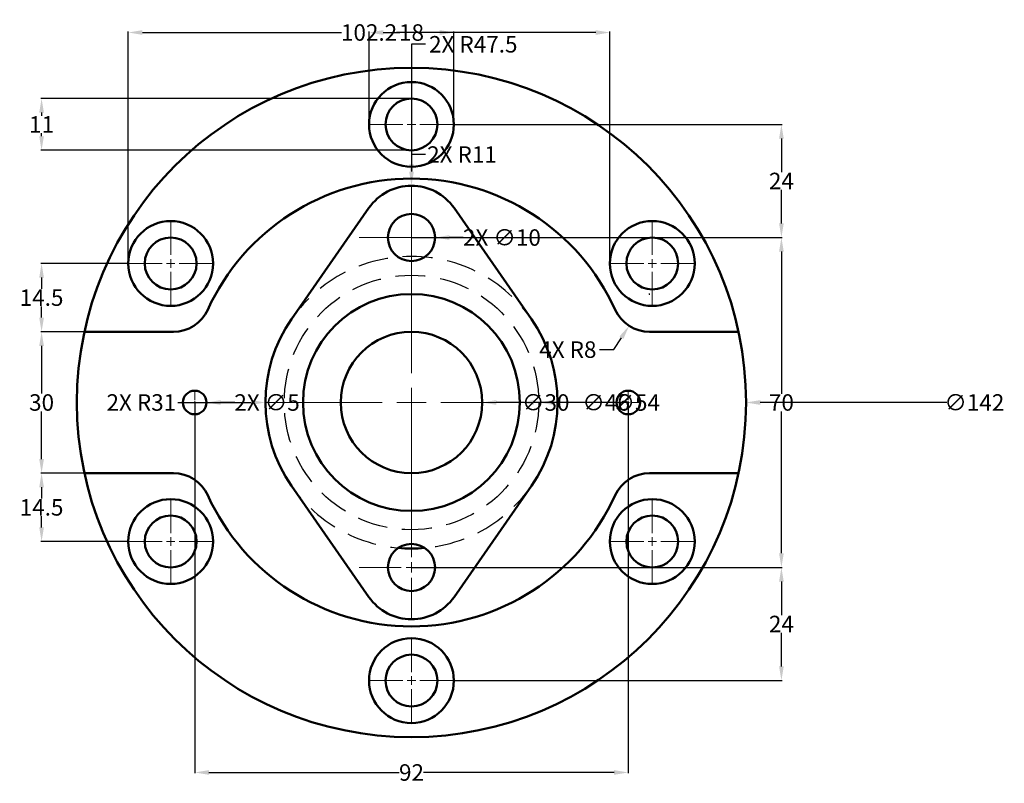
# Model space of a CAD drawing. Units: millimetres. Extents: x 646 to 860, y 238 to 552.
# Tile 2 of 2: x 651 to 860, y 390 to 552. Entities that reach past the tile are written whole.
import ezdxf

# ---------------------------------------------------------------- set-up
doc = ezdxf.new("R2010")
doc.units = ezdxf.units.MM
doc.header["$MEASUREMENT"] = 0
doc.linetypes.add('CENTER', pattern=[50.8, 31.75, -6.35, 6.35, -6.35])
doc.linetypes.add('HIDDEN', pattern=[9.525, 6.35, -3.175])
for name, color, linetype, lineweight in [('M-CNTR', 1, 'CENTER', 18), ('M-DIMS', 2, 'Continuous', 18), ('M-HIDN', 4, 'HIDDEN', 25), ('M-OUTL', 7, 'Continuous', 50)]:
    doc.layers.add(name, color=color, linetype=linetype, lineweight=lineweight)
doc.styles.get("Standard").update_dxf_attribs({"font": 'arial.ttf'})
doc.dimstyles.get("Standard").update_dxf_attribs({"dimtxt": 3.5, "dimasz": 3, "dimexe": 0.18, "dimexo": 0.0625, "dimgap": 0.09, "dimtad": 0, "dimtih": 1, "dimtoh": 1, "dimdec": 1, "dimzin": 0, "dimdsep": 46, "dimtxsty": 'Standard', "dimcen": 0.09, "dimadec": 0, "dimazin": 0, "dimtfac": 1, "dimtdec": 1, "dimtofl": 0, "dimtmove": 0, "dimatfit": 3, "dimfxl": 1, "dimtolj": 1, "dimtzin": 0, "dimarcsym": 0})

# ---------------------------------------------------------------- blocks, each defined once
blk = doc.blocks.new('*U1')
for radius in [9, 5.5]:
    blk.add_circle((0, 0), radius)
blk = doc.blocks.new('*U2')
at = {"layer": 'M-OUTL', "color": 0, "linetype": 'ByBlock', "lineweight": -2, "transparency": 16777216}
blk.add_blockref('*U1', (191, 167.28), dxfattribs=at)
for p, rotation in [((139.9, 137.78), 59.99999999999999), ((242.1, 137.78), 300), ((139.9, 78.78), 120), ((242.1, 78.78), 240), ((191, 49.28), 180)]:
    blk.add_blockref('*U1', p, dxfattribs=dict(at, rotation=rotation))
blk = doc.blocks.new('*U3')
at = {"layer": 'M-CNTR', "color": 0, "transparency": 16777216}
for p, q in [((0, 1.8), (0, 9.12)), ((-9.12, 0), (-1.8, 0)), ((1.8, 0), (9.12, 0)), ((0, -9.12), (0, -1.8))]:
    blk.add_line(p, q, dxfattribs=at)
at = {"layer": 'M-CNTR', "color": 0, "linetype": 'Continuous', "transparency": 16777216}
for p, q in [((-0.9, 0), (0.9, 0)), ((0, -0.9), (0, 0.9))]:
    blk.add_line(p, q, dxfattribs=at)
blk = doc.blocks.new('*U4')
at = {"layer": 'M-CNTR', "color": 0, "transparency": 16777216}
for p, q in [((0, 1.8), (0, 9.12)), ((-9.12, 0), (-1.8, 0)), ((1.8, 0), (9.12, 0)), ((0, -9.12), (0, -1.8))]:
    blk.add_line(p, q, dxfattribs=at)
at = {"layer": 'M-CNTR', "color": 0, "linetype": 'Continuous', "transparency": 16777216}
for p, q in [((-0.9, 0), (0.9, 0)), ((0, -0.9), (0, 0.9))]:
    blk.add_line(p, q, dxfattribs=at)
blk = doc.blocks.new('*U5')
at = {"layer": 'M-CNTR', "color": 0, "transparency": 16777216}
for p, q in [((0, 1.8), (0, 9.12)), ((-9.12, 0), (-1.8, 0)), ((1.8, 0), (9.12, 0)), ((0, -9.12), (0, -1.8))]:
    blk.add_line(p, q, dxfattribs=at)
at = {"layer": 'M-CNTR', "color": 0, "linetype": 'Continuous', "transparency": 16777216}
for p, q in [((-0.9, 0), (0.9, 0)), ((0, -0.9), (0, 0.9))]:
    blk.add_line(p, q, dxfattribs=at)
blk = doc.blocks.new('*U6')
at = {"layer": 'M-CNTR', "color": 0, "transparency": 16777216}
for p, q in [((0, 1.8), (0, 9.12)), ((-9.12, 0), (-1.8, 0)), ((1.8, 0), (9.12, 0)), ((0, -9.12), (0, -1.8))]:
    blk.add_line(p, q, dxfattribs=at)
at = {"layer": 'M-CNTR', "color": 0, "linetype": 'Continuous', "transparency": 16777216}
for p, q in [((-0.9, 0), (0.9, 0)), ((0, -0.9), (0, 0.9))]:
    blk.add_line(p, q, dxfattribs=at)
blk = doc.blocks.new('*U7')
at = {"layer": 'M-CNTR', "color": 0, "transparency": 16777216}
for p, q in [((0, 1.8), (0, 9.12)), ((-9.12, 0), (-1.8, 0)), ((1.8, 0), (9.12, 0)), ((0, -9.12), (0, -1.8))]:
    blk.add_line(p, q, dxfattribs=at)
at = {"layer": 'M-CNTR', "color": 0, "linetype": 'Continuous', "transparency": 16777216}
for p, q in [((-0.9, 0), (0.9, 0)), ((0, -0.9), (0, 0.9))]:
    blk.add_line(p, q, dxfattribs=at)
blk = doc.blocks.new('*U8')
at = {"layer": 'M-CNTR', "color": 0, "transparency": 16777216}
for p, q in [((0, 1.8), (0, 9.12)), ((-9.12, 0), (-1.8, 0)), ((1.8, 0), (9.12, 0)), ((0, -9.12), (0, -1.8))]:
    blk.add_line(p, q, dxfattribs=at)
at = {"layer": 'M-CNTR', "color": 0, "linetype": 'Continuous', "transparency": 16777216}
for p, q in [((-0.9, 0), (0.9, 0)), ((0, -0.9), (0, 0.9))]:
    blk.add_line(p, q, dxfattribs=at)
blk = doc.blocks.new('*U9')
at = {"layer": 'M-CNTR', "color": 0, "transparency": 16777216}
for p, q in [((0, 0.5), (0, 2.62)), ((-2.62, 0), (-0.5, 0)), ((0.5, 0), (2.62, 0)), ((0, -2.62), (0, -0.5))]:
    blk.add_line(p, q, dxfattribs=at)
at = {"layer": 'M-CNTR', "color": 0, "linetype": 'Continuous', "transparency": 16777216}
for p, q in [((-0.25, 0), (0.25, 0)), ((0, -0.25), (0, 0.25))]:
    blk.add_line(p, q, dxfattribs=at)
blk = doc.blocks.new('*U10')
at = {"layer": 'M-CNTR', "color": 0, "transparency": 16777216}
for p, q in [((0, 0.5), (0, 2.62)), ((-2.62, 0), (-0.5, 0)), ((0.5, 0), (2.62, 0)), ((0, -2.62), (0, -0.5))]:
    blk.add_line(p, q, dxfattribs=at)
at = {"layer": 'M-CNTR', "color": 0, "linetype": 'Continuous', "transparency": 16777216}
for p, q in [((-0.25, 0), (0.25, 0)), ((0, -0.25), (0, 0.25))]:
    blk.add_line(p, q, dxfattribs=at)
blk = doc.blocks.new('*U11')
at = {"layer": 'M-CNTR', "color": 0, "transparency": 16777216}
for p, q in [((0, 1), (0, 5.12)), ((-5.12, 0), (-1, 0)), ((1, 0), (5.12, 0)), ((0, -5.12), (0, -1))]:
    blk.add_line(p, q, dxfattribs=at)
at = {"layer": 'M-CNTR', "color": 0, "linetype": 'Continuous', "transparency": 16777216}
for p, q in [((-0.5, 0), (0.5, 0)), ((0, -0.5), (0, 0.5))]:
    blk.add_line(p, q, dxfattribs=at)
blk = doc.blocks.new('*U12')
at = {"layer": 'M-CNTR', "color": 0, "transparency": 16777216}
for p, q in [((0, 2.2), (0, 11.12)), ((-11.12, 0), (-2.2, 0)), ((2.2, 0), (11.12, 0)), ((0, -11.12), (0, -2.2))]:
    blk.add_line(p, q, dxfattribs=at)
at = {"layer": 'M-CNTR', "color": 0, "linetype": 'Continuous', "transparency": 16777216}
for p, q in [((-1.1, 0), (1.1, 0)), ((0, -1.1), (0, 1.1))]:
    blk.add_line(p, q, dxfattribs=at)
blk = doc.blocks.new('*U13')
at = {"layer": 'M-CNTR', "color": 0, "transparency": 16777216}
for p, q in [((0, 2.2), (0, 11.12)), ((-11.12, 0), (-2.2, 0)), ((2.2, 0), (11.12, 0)), ((0, -11.12), (0, -2.2))]:
    blk.add_line(p, q, dxfattribs=at)
at = {"layer": 'M-CNTR', "color": 0, "linetype": 'Continuous', "transparency": 16777216}
for p, q in [((-1.1, 0), (1.1, 0)), ((0, -1.1), (0, 1.1))]:
    blk.add_line(p, q, dxfattribs=at)
blk = doc.blocks.new('*U14')
at = {"layer": 'M-CNTR', "color": 0, "transparency": 16777216}
for p, q in [((0, 6.2), (0, 31.12)), ((-31.12, 0), (-6.2, 0)), ((6.2, 0), (31.12, 0)), ((0, -31.12), (0, -6.2))]:
    blk.add_line(p, q, dxfattribs=at)
at = {"layer": 'M-CNTR', "color": 0, "linetype": 'Continuous', "transparency": 16777216}
for p, q in [((0, -3.1), (0, 3.1)), ((-3.1, 0), (3.1, 0))]:
    blk.add_line(p, q, dxfattribs=at)
blk = doc.blocks.new('*D15')
at = {"layer": 'Defpoints', "color": 0, "transparency": 16777216}
for p in [(688.02, 471.16), (780.02, 471.16), (780.02, 392.66)]:
    blk.add_point(p, dxfattribs=at)
at = {"layer": 'M-DIMS', "color": 0, "lineweight": -2, "transparency": 16777216}
for p, q in [((688.02, 471.1), (688.02, 392.48)), ((780.02, 471.1), (780.02, 392.48)), ((691.02, 392.66), (731.44, 392.66)), ((777.02, 392.66), (736.59, 392.66))]:
    blk.add_line(p, q, dxfattribs=at)
at = {"layer": 'M-DIMS', "color": 0, "transparency": 16777216}
for points in [[(691.02, 393.16), (691.02, 392.16), (688.02, 392.66)], [(777.02, 393.16), (777.02, 392.16), (780.02, 392.66)]]:
    blk.add_solid(points, dxfattribs=at)
at = {"layer": 'M-DIMS', "color": 0, "transparency": 16777216, "insert": (734.02, 392.66), "char_height": 3.5, "attachment_point": 5}
blk.add_mtext('\\A1;92', dxfattribs=at)
blk = doc.blocks.new('*D16')
at = {"layer": 'Defpoints', "color": 0, "transparency": 16777216}
for p in [(743.02, 549.66), (725.02, 530.16), (743.02, 530.16)]:
    blk.add_point(p, dxfattribs=at)
at = {"layer": 'M-DIMS', "color": 0, "lineweight": -2, "transparency": 16777216}
for p, q in [((725.02, 530.22), (725.02, 549.84)), ((728.02, 549.66), (731.58, 549.66)), ((740.02, 549.66), (736.45, 549.66)), ((743.02, 530.22), (743.02, 549.84))]:
    blk.add_line(p, q, dxfattribs=at)
at = {"layer": 'M-DIMS', "color": 0, "transparency": 16777216}
for points in [[(728.02, 550.16), (728.02, 549.16), (725.02, 549.66)], [(740.02, 550.16), (740.02, 549.16), (743.02, 549.66)]]:
    blk.add_solid(points, dxfattribs=at)
at = {"layer": 'M-DIMS', "color": 0, "transparency": 16777216, "insert": (734.02, 549.66), "char_height": 3.5, "attachment_point": 5}
blk.add_mtext('\\A1;18', dxfattribs=at)
blk = doc.blocks.new('*D17')
at = {"layer": 'Defpoints', "color": 0, "transparency": 16777216}
for p in [(734.02, 535.66), (655.52, 524.66), (734.02, 524.66)]:
    blk.add_point(p, dxfattribs=at)
at = {"layer": 'M-DIMS', "color": 0, "lineweight": -2, "transparency": 16777216}
for p, q in [((733.95, 535.66), (655.34, 535.66)), ((655.52, 532.66), (655.52, 532.01)), ((655.52, 527.66), (655.52, 528.31)), ((733.95, 524.66), (655.34, 524.66))]:
    blk.add_line(p, q, dxfattribs=at)
at = {"layer": 'M-DIMS', "color": 0, "transparency": 16777216}
for points in [[(655.02, 532.66), (656.02, 532.66), (655.52, 535.66)], [(655.02, 527.66), (656.02, 527.66), (655.52, 524.66)]]:
    blk.add_solid(points, dxfattribs=at)
at = {"layer": 'M-DIMS', "color": 0, "transparency": 16777216, "insert": (655.52, 530.16), "char_height": 3.5, "attachment_point": 5}
blk.add_mtext('\\A1;11', dxfattribs=at)
blk = doc.blocks.new('*D18')
at = {"layer": 'Defpoints', "color": 0, "transparency": 16777216}
for p in [(776.11, 549.66), (673.92, 500.66), (776.11, 500.66)]:
    blk.add_point(p, dxfattribs=at)
at = {"layer": 'M-DIMS', "color": 0, "lineweight": -2, "transparency": 16777216}
for p, q in [((673.92, 500.72), (673.92, 549.84)), ((676.92, 549.66), (719.2, 549.66)), ((773.11, 549.66), (730.83, 549.66)), ((776.11, 500.72), (776.11, 549.84))]:
    blk.add_line(p, q, dxfattribs=at)
at = {"layer": 'M-DIMS', "color": 0, "transparency": 16777216}
for points in [[(676.92, 550.16), (676.92, 549.16), (673.92, 549.66)], [(773.11, 550.16), (773.11, 549.16), (776.11, 549.66)]]:
    blk.add_solid(points, dxfattribs=at)
at = {"layer": 'M-DIMS', "color": 0, "transparency": 16777216, "insert": (725.02, 549.66), "char_height": 3.5, "attachment_point": 5}
blk.add_mtext('\\A1;102.2', dxfattribs=at)
blk = doc.blocks.new('*D19')
at = {"layer": 'Defpoints', "color": 0, "transparency": 16777216}
for p in [(655.52, 456.16), (664.62, 456.16), (673.92, 441.66)]:
    blk.add_point(p, dxfattribs=at)
at = {"layer": 'M-DIMS', "color": 0, "lineweight": -2, "transparency": 16777216}
for p, q in [((664.56, 456.16), (655.34, 456.16)), ((655.52, 453.16), (655.52, 450.78)), ((655.52, 444.66), (655.52, 447.03)), ((673.86, 441.66), (655.34, 441.66))]:
    blk.add_line(p, q, dxfattribs=at)
at = {"layer": 'M-DIMS', "color": 0, "transparency": 16777216}
for points in [[(655.02, 453.16), (656.02, 453.16), (655.52, 456.16)], [(655.02, 444.66), (656.02, 444.66), (655.52, 441.66)]]:
    blk.add_solid(points, dxfattribs=at)
at = {"layer": 'M-DIMS', "color": 0, "transparency": 16777216, "insert": (655.52, 448.91), "char_height": 3.5, "attachment_point": 5}
blk.add_mtext('\\A1;14.5', dxfattribs=at)
blk = doc.blocks.new('*D20')
at = {"layer": 'Defpoints', "color": 0, "transparency": 16777216}
for p in [(655.52, 486.16), (664.62, 486.16), (664.62, 456.16)]:
    blk.add_point(p, dxfattribs=at)
at = {"layer": 'M-DIMS', "color": 0, "lineweight": -2, "transparency": 16777216}
for p, q in [((664.56, 486.16), (655.34, 486.16)), ((655.52, 483.16), (655.52, 473.04)), ((655.52, 459.16), (655.52, 469.28)), ((664.56, 456.16), (655.34, 456.16))]:
    blk.add_line(p, q, dxfattribs=at)
at = {"layer": 'M-DIMS', "color": 0, "transparency": 16777216}
for points in [[(655.02, 483.16), (656.02, 483.16), (655.52, 486.16)], [(655.02, 459.16), (656.02, 459.16), (655.52, 456.16)]]:
    blk.add_solid(points, dxfattribs=at)
at = {"layer": 'M-DIMS', "color": 0, "transparency": 16777216, "insert": (655.52, 471.16), "char_height": 3.5, "attachment_point": 5}
blk.add_mtext('\\A1;30', dxfattribs=at)
blk = doc.blocks.new('*D21')
at = {"layer": 'Defpoints', "color": 0, "transparency": 16777216}
for p in [(655.52, 500.66), (673.92, 500.66), (664.62, 486.16)]:
    blk.add_point(p, dxfattribs=at)
at = {"layer": 'M-DIMS', "color": 0, "lineweight": -2, "transparency": 16777216}
for p, q in [((673.86, 500.66), (655.34, 500.66)), ((655.52, 497.66), (655.52, 495.28)), ((655.52, 489.16), (655.52, 491.53)), ((664.56, 486.16), (655.34, 486.16))]:
    blk.add_line(p, q, dxfattribs=at)
at = {"layer": 'M-DIMS', "color": 0, "transparency": 16777216}
for points in [[(655.02, 497.66), (656.02, 497.66), (655.52, 500.66)], [(655.02, 489.16), (656.02, 489.16), (655.52, 486.16)]]:
    blk.add_solid(points, dxfattribs=at)
at = {"layer": 'M-DIMS', "color": 0, "transparency": 16777216, "insert": (655.52, 493.41), "char_height": 3.5, "attachment_point": 5}
blk.add_mtext('\\A1;14.5', dxfattribs=at)
blk = doc.blocks.new('*D22')
at = {"layer": 'Defpoints', "color": 0, "transparency": 16777216}
for p in [(734.02, 436.16), (812.52, 436.16), (743.02, 412.16)]:
    blk.add_point(p, dxfattribs=at)
at = {"layer": 'M-DIMS', "color": 0, "lineweight": -2, "transparency": 16777216}
for p, q in [((734.08, 436.16), (812.7, 436.16)), ((812.52, 433.16), (812.52, 426.01)), ((812.52, 415.16), (812.52, 422.31)), ((743.08, 412.16), (812.7, 412.16))]:
    blk.add_line(p, q, dxfattribs=at)
at = {"layer": 'M-DIMS', "color": 0, "transparency": 16777216}
for points in [[(812.02, 433.16), (813.02, 433.16), (812.52, 436.16)], [(812.02, 415.16), (813.02, 415.16), (812.52, 412.16)]]:
    blk.add_solid(points, dxfattribs=at)
at = {"layer": 'M-DIMS', "color": 0, "transparency": 16777216, "insert": (812.52, 424.16), "char_height": 3.5, "attachment_point": 5}
blk.add_mtext('\\A1;24', dxfattribs=at)
blk = doc.blocks.new('*D23')
at = {"layer": 'Defpoints', "color": 0, "transparency": 16777216}
for p in [(734.02, 506.16), (812.52, 506.16), (734.02, 436.16)]:
    blk.add_point(p, dxfattribs=at)
at = {"layer": 'M-DIMS', "color": 0, "lineweight": -2, "transparency": 16777216}
for p, q in [((734.08, 506.16), (812.7, 506.16)), ((812.52, 503.16), (812.52, 473.03)), ((812.52, 439.16), (812.52, 469.28)), ((734.08, 436.16), (812.7, 436.16))]:
    blk.add_line(p, q, dxfattribs=at)
at = {"layer": 'M-DIMS', "color": 0, "transparency": 16777216}
for points in [[(812.02, 503.16), (813.02, 503.16), (812.52, 506.16)], [(812.02, 439.16), (813.02, 439.16), (812.52, 436.16)]]:
    blk.add_solid(points, dxfattribs=at)
at = {"layer": 'M-DIMS', "color": 0, "transparency": 16777216, "insert": (812.52, 471.16), "char_height": 3.5, "attachment_point": 5}
blk.add_mtext('\\A1;70', dxfattribs=at)
blk = doc.blocks.new('*D24')
at = {"layer": 'Defpoints', "color": 0, "transparency": 16777216}
for p in [(743.02, 530.16), (812.52, 530.16), (734.02, 506.16)]:
    blk.add_point(p, dxfattribs=at)
at = {"layer": 'M-DIMS', "color": 0, "lineweight": -2, "transparency": 16777216}
for p, q in [((743.08, 530.16), (812.7, 530.16)), ((812.52, 527.16), (812.52, 520.01)), ((812.52, 509.16), (812.52, 516.31)), ((734.08, 506.16), (812.7, 506.16))]:
    blk.add_line(p, q, dxfattribs=at)
at = {"layer": 'M-DIMS', "color": 0, "transparency": 16777216}
for points in [[(812.02, 527.16), (813.02, 527.16), (812.52, 530.16)], [(812.02, 509.16), (813.02, 509.16), (812.52, 506.16)]]:
    blk.add_solid(points, dxfattribs=at)
at = {"layer": 'M-DIMS', "color": 0, "transparency": 16777216, "insert": (812.52, 518.16), "char_height": 3.5, "attachment_point": 5}
blk.add_mtext('\\A1;24', dxfattribs=at)
blk = doc.blocks.new('*D40')
at = {"layer": 'Defpoints', "color": 0, "transparency": 16777216}
for p in [(663.02, 471.16), (805.02, 471.16)]:
    blk.add_point(p, dxfattribs=at)
at = {"layer": 'M-DIMS', "color": 0, "lineweight": -2, "transparency": 16777216}
for p, q in [((733.93, 471.16), (734.11, 471.16)), ((734.02, 471.07), (734.02, 471.25)), ((847.62, 471.16), (808.02, 471.16))]:
    blk.add_line(p, q, dxfattribs=at)
at = {"layer": 'M-DIMS', "color": 0, "transparency": 16777216}
blk.add_solid([(808.02, 471.66), (808.02, 470.66), (805.02, 471.16)], dxfattribs=at)
at = {"layer": 'M-DIMS', "color": 0, "transparency": 16777216, "insert": (853.46, 471.16), "char_height": 3.5, "attachment_point": 5}
blk.add_mtext('\\A1;∅142', dxfattribs=at)
blk = doc.blocks.new('*D41')
at = {"layer": 'Defpoints', "color": 0, "transparency": 16777216}
for p in [(734.02, 518.66), (734.02, 471.16)]:
    blk.add_point(p, dxfattribs=at)
at = {"layer": 'M-DIMS', "color": 0, "lineweight": -2, "transparency": 16777216}
for p, q in [((737.02, 547.16), (734.02, 547.16)), ((734.02, 547.16), (734.02, 521.66)), ((733.93, 471.16), (734.11, 471.16)), ((734.02, 471.07), (734.02, 471.25))]:
    blk.add_line(p, q, dxfattribs=at)
at = {"layer": 'M-DIMS', "color": 0, "transparency": 16777216}
blk.add_solid([(733.52, 521.66), (734.52, 521.66), (734.02, 518.66)], dxfattribs=at)
at = {"layer": 'M-DIMS', "color": 0, "transparency": 16777216, "insert": (747.13, 547.16), "char_height": 3.5, "attachment_point": 5}
blk.add_mtext('\\A1;2X R47.5', dxfattribs=at)
blk = doc.blocks.new('*D42')
at = {"layer": 'Defpoints', "color": 0, "transparency": 16777216}
for p in [(784.53, 494.16), (780.2, 487.43)]:
    blk.add_point(p, dxfattribs=at)
at = {"layer": 'M-DIMS', "color": 0, "lineweight": -2, "transparency": 16777216}
for p, q in [((784.44, 494.16), (784.62, 494.16)), ((784.53, 494.07), (784.53, 494.25)), ((776.95, 482.38), (778.57, 484.91)), ((773.95, 482.38), (776.95, 482.38))]:
    blk.add_line(p, q, dxfattribs=at)
at = {"layer": 'M-DIMS', "color": 0, "transparency": 16777216}
blk.add_solid([(778.15, 485.18), (778.99, 484.64), (780.2, 487.43)], dxfattribs=at)
at = {"layer": 'M-DIMS', "color": 0, "transparency": 16777216, "insert": (767.2, 482.38), "char_height": 3.5, "attachment_point": 5}
blk.add_mtext('\\A1;4X R8', dxfattribs=at)
blk = doc.blocks.new('*D43')
at = {"layer": 'Defpoints', "color": 0, "transparency": 16777216}
for p in [(703.02, 471.16), (734.02, 471.16)]:
    blk.add_point(p, dxfattribs=at)
at = {"layer": 'M-DIMS', "color": 0, "lineweight": -2, "transparency": 16777216}
for p, q in [((684.42, 471.16), (700.02, 471.16)), ((733.93, 471.16), (734.11, 471.16)), ((734.02, 471.07), (734.02, 471.25))]:
    blk.add_line(p, q, dxfattribs=at)
at = {"layer": 'M-DIMS', "color": 0, "transparency": 16777216}
blk.add_solid([(700.02, 471.66), (700.02, 470.66), (703.02, 471.16)], dxfattribs=at)
at = {"layer": 'M-DIMS', "color": 0, "transparency": 16777216, "insert": (676.69, 471.16), "char_height": 3.5, "attachment_point": 5}
blk.add_mtext('\\A1;2X R31', dxfattribs=at)
blk = doc.blocks.new('*D44')
at = {"layer": 'Defpoints', "color": 0, "transparency": 16777216}
for p in [(734.02, 517.16), (734.02, 506.16)]:
    blk.add_point(p, dxfattribs=at)
at = {"layer": 'M-DIMS', "color": 0, "lineweight": -2, "transparency": 16777216}
for p, q in [((737.02, 523.76), (734.02, 523.76)), ((734.02, 523.76), (734.02, 520.16)), ((733.93, 506.16), (734.11, 506.16)), ((734.02, 506.07), (734.02, 506.25))]:
    blk.add_line(p, q, dxfattribs=at)
at = {"layer": 'M-DIMS', "color": 0, "transparency": 16777216}
blk.add_solid([(733.52, 520.16), (734.52, 520.16), (734.02, 517.16)], dxfattribs=at)
at = {"layer": 'M-DIMS', "color": 0, "transparency": 16777216, "insert": (744.74, 523.76), "char_height": 3.5, "attachment_point": 5}
blk.add_mtext('\\A1;2X R11', dxfattribs=at)
blk = doc.blocks.new('*D45')
at = {"layer": 'Defpoints', "color": 0, "transparency": 16777216}
for p in [(729.02, 506.16), (739.02, 506.16)]:
    blk.add_point(p, dxfattribs=at)
at = {"layer": 'M-DIMS', "color": 0, "lineweight": -2, "transparency": 16777216}
for p, q in [((733.93, 506.16), (734.11, 506.16)), ((734.02, 506.07), (734.02, 506.25)), ((745.02, 506.16), (742.02, 506.16))]:
    blk.add_line(p, q, dxfattribs=at)
at = {"layer": 'M-DIMS', "color": 0, "transparency": 16777216}
blk.add_solid([(742.02, 506.66), (742.02, 505.66), (739.02, 506.16)], dxfattribs=at)
at = {"layer": 'M-DIMS', "color": 0, "transparency": 16777216, "insert": (753.21, 506.16), "char_height": 3.5, "attachment_point": 5}
blk.add_mtext('\\A1;2X ∅10', dxfattribs=at)
blk = doc.blocks.new('*D46')
at = {"layer": 'Defpoints', "color": 0, "transparency": 16777216}
for p in [(685.52, 471.16), (690.52, 471.16)]:
    blk.add_point(p, dxfattribs=at)
at = {"layer": 'M-DIMS', "color": 0, "lineweight": -2, "transparency": 16777216}
for p, q in [((687.93, 471.16), (688.11, 471.16)), ((688.02, 471.07), (688.02, 471.25)), ((696.52, 471.16), (693.52, 471.16))]:
    blk.add_line(p, q, dxfattribs=at)
at = {"layer": 'M-DIMS', "color": 0, "transparency": 16777216}
blk.add_solid([(693.52, 471.66), (693.52, 470.66), (690.52, 471.16)], dxfattribs=at)
at = {"layer": 'M-DIMS', "color": 0, "transparency": 16777216, "insert": (703.37, 471.16), "char_height": 3.5, "attachment_point": 5}
blk.add_mtext('\\A1;2X ∅5', dxfattribs=at)
blk = doc.blocks.new('*D47')
at = {"layer": 'Defpoints', "color": 0, "transparency": 16777216}
for p in [(711.02, 471.16), (757.02, 471.16)]:
    blk.add_point(p, dxfattribs=at)
at = {"layer": 'M-DIMS', "color": 0, "lineweight": -2, "transparency": 16777216}
for p, q in [((733.93, 471.16), (734.11, 471.16)), ((734.02, 471.07), (734.02, 471.25)), ((770.82, 471.16), (760.02, 471.16))]:
    blk.add_line(p, q, dxfattribs=at)
at = {"layer": 'M-DIMS', "color": 0, "transparency": 16777216}
blk.add_solid([(760.02, 471.66), (760.02, 470.66), (757.02, 471.16)], dxfattribs=at)
at = {"layer": 'M-DIMS', "color": 0, "transparency": 16777216, "insert": (775.32, 471.16), "char_height": 3.5, "attachment_point": 5}
blk.add_mtext('\\A1;∅46', dxfattribs=at)
blk = doc.blocks.new('*D48')
at = {"layer": 'Defpoints', "color": 0, "transparency": 16777216}
for p in [(719.02, 471.16), (749.02, 471.16)]:
    blk.add_point(p, dxfattribs=at)
at = {"layer": 'M-DIMS', "color": 0, "lineweight": -2, "transparency": 16777216}
for p, q in [((733.93, 471.16), (734.11, 471.16)), ((734.02, 471.07), (734.02, 471.25)), ((758.02, 471.16), (752.02, 471.16))]:
    blk.add_line(p, q, dxfattribs=at)
at = {"layer": 'M-DIMS', "color": 0, "transparency": 16777216}
blk.add_solid([(752.02, 471.66), (752.02, 470.66), (749.02, 471.16)], dxfattribs=at)
at = {"layer": 'M-DIMS', "color": 0, "transparency": 16777216, "insert": (762.51, 471.16), "char_height": 3.5, "attachment_point": 5}
blk.add_mtext('\\A1;∅30', dxfattribs=at)
blk = doc.blocks.new('*D49')
at = {"layer": 'Defpoints', "color": 0, "transparency": 16777216}
for p in [(707.02, 471.16), (761.02, 471.16)]:
    blk.add_point(p, dxfattribs=at)
at = {"layer": 'M-DIMS', "color": 0, "lineweight": -2, "transparency": 16777216}
for p, q in [((733.93, 471.16), (734.11, 471.16)), ((734.02, 471.07), (734.02, 471.25)), ((777.22, 471.16), (764.02, 471.16))]:
    blk.add_line(p, q, dxfattribs=at)
at = {"layer": 'M-DIMS', "color": 0, "transparency": 16777216}
blk.add_solid([(764.02, 471.66), (764.02, 470.66), (761.02, 471.16)], dxfattribs=at)
at = {"layer": 'M-DIMS', "color": 0, "transparency": 16777216, "insert": (781.71, 471.16), "char_height": 3.5, "attachment_point": 5}
blk.add_mtext('\\A1;∅54', dxfattribs=at)

msp = doc.modelspace()

# ---------------------------------------------------------------- linework, layer by layer
at = {"layer": 'M-CNTR'}
msp.add_line((734.016, 471.158), (734.016, 436.158), dxfattribs=at)
at = {"layer": 'M-HIDN'}
msp.add_circle((734.016, 471.158), 27, dxfattribs=at)
for start, end in [(28.93853, 151.06147), (208.93853, 331.06147)]:
    msp.add_arc((734.016, 471.158), 31, start, end, dxfattribs=at)
at = {"layer": 'M-OUTL'}
for p, q in [((724.989, 512.444), (708.576, 488.872)), ((743.043, 512.444), (759.456, 488.872)), ((683.506, 486.158), (664.618, 486.158)), ((803.413, 486.158), (784.526, 486.158)), ((683.506, 456.158), (664.618, 456.158)), ((803.413, 456.158), (784.526, 456.158)), ((724.989, 429.872), (708.576, 453.444)), ((743.043, 429.872), (759.456, 453.444))]:
    msp.add_line(p, q, dxfattribs=at)
for centre, radius in [((734.016, 471.158), 71), ((734.016, 506.158), 5), ((734.016, 471.158), 23), ((734.016, 471.158), 15), ((688.016, 471.158), 2.5), ((780.016, 471.158), 2.5), ((734.016, 436.158), 5)]:
    msp.add_circle(centre, radius, dxfattribs=at)
for centre, radius, start, end in [((734.016, 471.158), 47.5, 24.48244, 155.51756), ((734.016, 506.158), 11, 34.8499, 145.1501), ((683.506, 494.158), 8, 270, 335.51756), ((784.526, 494.158), 8, 204.48244, 270), ((734.016, 471.158), 31, 145.1501, 214.8499), ((734.016, 471.158), 31, 325.1501, 34.8499), ((683.506, 448.158), 8, 24.48244, 90), ((784.526, 448.158), 8, 90, 155.51756), ((734.016, 471.158), 47.5, 204.48244, 335.51756), ((734.016, 471.158), 31, 264.7799, 275.2201), ((734.016, 436.158), 11, 214.8499, 325.1501)]:
    msp.add_arc(centre, radius, start, end, dxfattribs=at)

# ---------------------------------------------------------------- block references
at = {"layer": 'M-CNTR'}
for name, p in [('*U3', (734.016, 530.158)), ('*U12', (734.016, 506.158)), ('*U11', (734.016, 506.158)), ('*U5', (682.92, 500.658)), ('*U4', (785.111, 500.658)), ('*U14', (734.016, 471.158)), ('*U10', (688.016, 471.158)), ('*U9', (780.016, 471.158)), ('*U6', (682.92, 441.658)), ('*U8', (785.111, 441.658)), ('*U13', (734.016, 436.158)), ('*U7', (734.016, 412.158))]:
    msp.add_blockref(name, p, dxfattribs=at)
at = {"layer": 'M-OUTL'}
msp.add_blockref('*U2', (543.016, 362.875), dxfattribs=at)

# ---------------------------------------------------------------- dimensions: what is measured, and where the dimension line sits
at = {"layer": 'M-DIMS'}
for base, p1, p2, override, picture, middle in [((776.111, 549.658), (673.92, 500.658), (776.111, 500.658), {"dimdec": 1, "dimlfac": 1, "dimrnd": 0, "dimzin": 0, "dimdsep": 46, "dimlunit": 2}, '*D18', (725.016, 549.658)), ((743.016, 549.658), (725.016, 530.158), (743.016, 530.158), {"dimdec": 0, "dimlfac": 1, "dimrnd": 0, "dimzin": 0, "dimdsep": 46, "dimlunit": 2}, '*D16', (734.016, 549.658)), ((780.016, 392.658), (688.016, 471.158), (780.016, 471.158), {"dimdec": 0, "dimlfac": 1, "dimrnd": 0, "dimzin": 0, "dimdsep": 46, "dimlunit": 2}, '*D15', (734.016, 392.658))]:
    dim = msp.add_linear_dim(base=base, p1=p1, p2=p2, dimstyle='Standard', override=override, dxfattribs=at)
    dim.commit()
    dim.dimension.update_dxf_attribs({"geometry": picture, "text_midpoint": middle})
for center, mpoint, override, picture, middle in [((734.016, 471.158), (734.016, 518.658), {"dimdec": 1, "dimlfac": 1, "dimrnd": 0, "dimzin": 0, "dimdsep": 46, "dimlunit": 2}, '*D41', (747.13, 547.158)), ((734.016, 506.158), (734.016, 517.158), {"dimdec": 0, "dimlfac": 1, "dimrnd": 0, "dimzin": 0, "dimdsep": 46, "dimlunit": 2}, '*D44', (744.74, 523.758)), ((734.016, 471.158), (703.016, 471.158), {"dimdec": 0, "dimlfac": 1, "dimrnd": 0, "dimzin": 0, "dimdsep": 46, "dimlunit": 2}, '*D43', (684.416, 471.158))]:
    dim = msp.add_radius_dim(center=center, mpoint=mpoint, text='2X <>', dimstyle='Standard', override=override, dxfattribs=at)
    dim.commit()
    dim.dimension.update_dxf_attribs({"geometry": picture, "text_midpoint": middle, "dimtype": 164})
for base, p1, p2, override, picture, middle in [((655.516, 524.658), (734.016, 535.658), (734.016, 524.658), {"dimdec": 0, "dimlfac": 1, "dimrnd": 0, "dimzin": 0, "dimdsep": 46, "dimlunit": 2}, '*D17', (655.516, 530.158)), ((812.516, 530.158), (734.016, 506.158), (743.016, 530.158), {"dimdec": 0, "dimlfac": 1, "dimrnd": 0, "dimzin": 0, "dimdsep": 46, "dimlunit": 2}, '*D24', (812.516, 518.158)), ((812.516, 506.158), (734.016, 436.158), (734.016, 506.158), {"dimdec": 0, "dimlfac": 1, "dimrnd": 0, "dimzin": 0, "dimdsep": 46, "dimlunit": 2}, '*D23', (812.516, 471.158)), ((655.516, 500.658), (664.618, 486.158), (673.92, 500.658), {"dimdec": 1, "dimlfac": 1, "dimrnd": 0, "dimzin": 0, "dimdsep": 46, "dimlunit": 2}, '*D21', (655.516, 493.408)), ((655.516, 486.158), (664.618, 456.158), (664.618, 486.158), {"dimdec": 0, "dimlfac": 1, "dimrnd": 0, "dimzin": 0, "dimdsep": 46, "dimlunit": 2}, '*D20', (655.516, 471.158)), ((655.516, 456.158), (673.92, 441.658), (664.618, 456.158), {"dimdec": 1, "dimlfac": 1, "dimrnd": 0, "dimzin": 0, "dimdsep": 46, "dimlunit": 2}, '*D19', (655.516, 448.908)), ((812.516, 436.158), (743.016, 412.158), (734.016, 436.158), {"dimdec": 0, "dimlfac": 1, "dimrnd": 0, "dimzin": 0, "dimdsep": 46, "dimlunit": 2}, '*D22', (812.516, 424.158))]:
    dim = msp.add_linear_dim(base=base, p1=p1, p2=p2, angle=90, dimstyle='Standard', override=override, dxfattribs=at)
    dim.commit()
    dim.dimension.update_dxf_attribs({"geometry": picture, "text_midpoint": middle})
for p1, p2, picture, middle in [((729.016, 506.158), (739.016, 506.158), '*D45', (745.016, 506.158)), ((685.516, 471.158), (690.516, 471.158), '*D46', (696.516, 471.158))]:
    dim = msp.add_diameter_dim_2p(p1=p1, p2=p2, text='2X <>', dimstyle='Standard', override={"dimdec": 0, "dimlfac": 1, "dimrnd": 0, "dimzin": 0, "dimdsep": 46, "dimlunit": 2}, dxfattribs=at)
    dim.commit()
    dim.dimension.update_dxf_attribs({"geometry": picture, "text_midpoint": middle, "dimtype": 163})
dim = msp.add_radius_dim(center=(784.526, 494.158), mpoint=(780.197, 487.43), text='4X <>', dimstyle='Standard', override={"dimdec": 0, "dimlfac": 1, "dimrnd": 0, "dimzin": 0, "dimdsep": 46, "dimlunit": 2}, dxfattribs=at)
dim.commit()
dim.dimension.update_dxf_attribs({"geometry": '*D42', "text_midpoint": (767.204, 482.384)})
for p1, p2, picture, middle in [((663.016, 471.158), (805.016, 471.158), '*D40', (847.616, 471.158)), ((707.016, 471.158), (761.016, 471.158), '*D49', (777.216, 471.158)), ((711.016, 471.158), (757.016, 471.158), '*D47', (770.816, 471.158)), ((719.016, 471.158), (749.016, 471.158), '*D48', (758.016, 471.158))]:
    dim = msp.add_diameter_dim_2p(p1=p1, p2=p2, dimstyle='Standard', override={"dimdec": 0, "dimlfac": 1, "dimrnd": 0, "dimzin": 0, "dimdsep": 46, "dimlunit": 2}, dxfattribs=at)
    dim.commit()
    dim.dimension.update_dxf_attribs({"geometry": picture, "text_midpoint": middle, "dimtype": 163})

doc.saveas('drawing.dxf')
